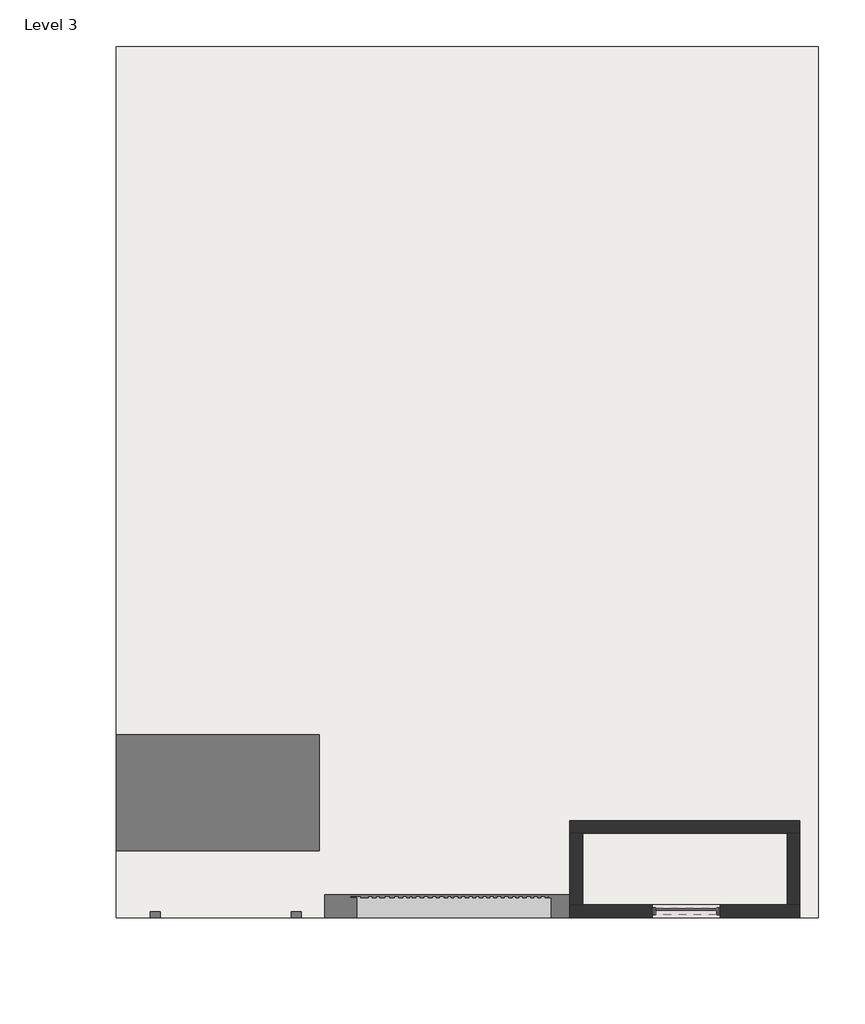
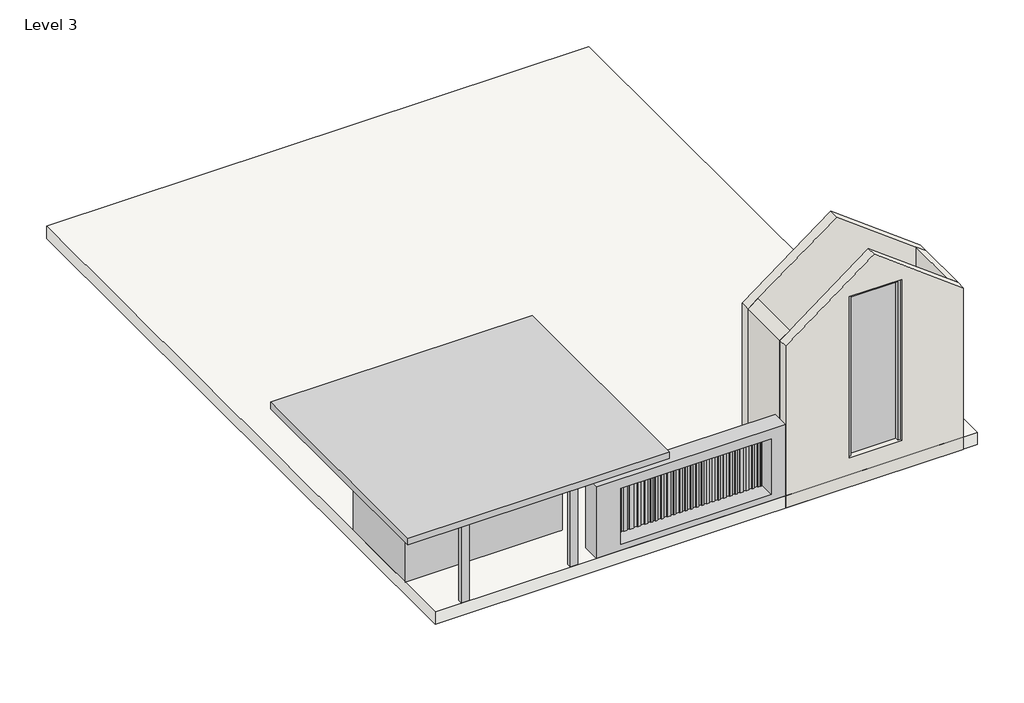
# One storey: 4 walls, 3 members, 1 plate, 1 proxy, 1 roof.
"""IFC4 building model written with IfcOpenShell, lengths in millimetres."""

from ifc_helpers import new_model, si_unit, frame, origin, place, context, project, spatial, polyline, outline, extrude, faceted_brep, transform, mapped, element, save
from components import generic_models_5_generic_models_5_ad9e1d00, member_97fca31a, member_273a15f2, system_panel_glazed_cfc6ab68

model = new_model("IFC4")

# Units and contexts
model_context = context("Model", 3, world=origin())
ifc_project = project(units=[si_unit("LENGTHUNIT", "METRE", prefix="MILLI")], contexts=[model_context])

# Site, building, storey
site = spatial("IfcSite", under=ifc_project)
building = spatial("IfcBuilding", under=site)
storey = spatial("IfcBuildingStorey", under=building, Name="Level 3", Elevation=6096.0)

# Proxy
placement = place(None, origin())
generic_models_5_generic_models_5_shape = generic_models_5_generic_models_5_ad9e1d00(model_context)
element("IfcBuildingElementProxy", 1, Name="Generic Models 5 : Generic Models 5", ObjectType="Generic Models 5 : Generic Models 5", at=placement, inside=storey, context=model_context, shape_type="MappedRepresentation", body=[
    mapped(generic_models_5_generic_models_5_shape, transform((0.0, 0.0, 0.0), x_axis=(1.0, 0.0, 0.0), y_axis=(0.0, 1.0, 0.0), z_axis=(0.0, 0.0, 1.0))),
])

# Members
member_shape = member_97fca31a(model_context)
element("IfcMember", 2, ObjectType="Rectangular Mullion : 2.5\" x 5\" rectangular", at=placement, inside=storey, context=model_context, shape_type="MappedRepresentation", body=[
    mapped(member_shape, transform((-12184.4451697, -14789.9171312, 10792.4603999), x_axis=(-1.0, 0.0, 0.0), y_axis=(0.0, -1.0, 0.0), z_axis=(0.0, 0.0, 1.0))),
])
member_2_shape = member_273a15f2(model_context)
element("IfcMember", 3, ObjectType="Rectangular Mullion : 2.5\" x 5\" rectangular", at=placement, inside=storey, context=model_context, shape_type="MappedRepresentation", body=[
    mapped(member_2_shape, transform((-11028.7451697, -14789.9171312, 10792.4603999), x_axis=(0.0, 0.0, 1.0), y_axis=(0.0, -1.0, 0.0), z_axis=(1.0, 0.0, 0.0))),
])
element("IfcMember", 4, ObjectType="Rectangular Mullion : 2.5\" x 5\" rectangular", at=placement, inside=storey, context=model_context, shape_type="MappedRepresentation", body=[
    mapped(member_shape, transform((-10965.2451697, -14789.9171312, 6813.0609972), x_axis=(1.0, 0.0, 0.0), y_axis=(0.0, -1.0, 0.0), z_axis=(0.0, 0.0, -1.0))),
])

# Plate
system_panel_glazed_shape = system_panel_glazed_cfc6ab68(model_context)
element("IfcPlate", 5, ObjectType="System Panel : Glazed", at=placement, inside=storey, context=model_context, shape_type="MappedRepresentation", body=[
    mapped(system_panel_glazed_shape, transform((-11574.8451697, -14789.9171312, 6813.0609972), x_axis=(1.0, 0.0, 0.0), y_axis=(0.0, 1.0, 0.0), z_axis=(0.0, 0.0, 1.0))),
])

# Roof
element("IfcRoof", 6, ObjectType="Generic - 12\"", at=placement, inside=storey, context=model_context, shape_type="SweptSolid", body=[
    extrude(outline(polyline([(-21845.6161422, 792.9828688), (-9196.4161422, 792.9828688), (-9196.4161422, -14904.2171312), (-21845.6161422, -14904.2171312), (-21845.6161422, 792.9828688)])), frame((0.0, 0.0, 6096.0), z_axis=(0.0, 0.0, 1.0), x_axis=(1.0, 0.0, 0.0)), (0.0, 0.0, 1.0), 304.8),
])

# Walls
element("IfcWall", 7, ObjectType="9\"", at=placement, inside=storey, context=model_context, shape_type="Brep", body=[
    faceted_brep([(-9528.1904814, -13160.519515, 6096.0), (-13670.3451697, -13160.519515, 6096.0), (-13670.3451697, -13160.519515, 10093.0339489), (-11606.7483033, -13160.519515, 11640.7315987), (-9528.1904814, -13160.519515, 10081.8132324), (-9528.1904814, -13389.119515, 6096.0), (-9528.1904814, -13389.119515, 10081.8132324), (-9756.7904814, -13389.119515, 10253.2632324), (-11606.7483033, -13389.119515, 11640.7315987), (-13441.7451697, -13389.119515, 10264.4839489), (-13670.3451697, -13389.119515, 10093.0339489), (-13670.3451697, -13389.119515, 6096.0), (-13441.7451697, -13389.119515, 6096.0), (-9756.7904814, -13389.119515, 6096.0)], [[[0, 1, 2, 3, 4]], [[5, 6, 7, 8, 9, 10, 11, 12, 13]], [[1, 0, 5, 13, 12, 11]], [[0, 4, 6, 5]], [[2, 1, 11, 10]], [[4, 3, 8, 7, 6]], [[3, 2, 10, 9, 8]]]),
])
element("IfcWall", 8, ObjectType="9\"", at=placement, inside=storey, context=model_context, shape_type="Brep", body=[
    faceted_brep([(-13670.3451697, -14904.2171312, 6096.0), (-9528.1904814, -14904.2171312, 6096.0), (-9528.1904814, -14904.2171312, 10081.8132324), (-11606.7483033, -14904.2171312, 11640.7315987), (-13670.3451697, -14904.2171312, 10093.0339489), (-12184.4451697, -14904.2171312, 6813.0609972), (-12184.4451697, -14904.2171312, 10792.4603999), (-10965.2451697, -14904.2171312, 10792.4603999), (-10965.2451697, -14904.2171312, 6813.0609972), (-9528.1904814, -14675.6171312, 6096.0), (-9756.7904814, -14675.6171312, 6096.0), (-13441.7451697, -14675.6171312, 6096.0), (-13670.3451697, -14675.6171312, 6096.0), (-13670.3451697, -14675.6171312, 10093.0339489), (-13441.7451697, -14675.6171312, 10264.4839489), (-11606.7483033, -14675.6171312, 11640.7315987), (-9756.7904814, -14675.6171312, 10253.2632324), (-9528.1904814, -14675.6171312, 10081.8132324), (-12184.4451697, -14675.6171312, 10792.4603999), (-12184.4451697, -14675.6171312, 6813.0609972), (-10965.2451697, -14675.6171312, 6813.0609972), (-10965.2451697, -14675.6171312, 10792.4603999)], [[[0, 1, 2, 3, 4], [5, 6, 7, 8]], [[9, 10, 11, 12, 13, 14, 15, 16, 17], [18, 19, 20, 21]], [[2, 1, 9, 17]], [[1, 0, 12, 11, 10, 9]], [[0, 4, 13, 12]], [[13, 4, 3, 15, 14]], [[2, 17, 16, 15, 3]], [[5, 19, 18, 6]], [[6, 18, 21, 7]], [[7, 21, 20, 8]], [[19, 5, 8, 20]]]),
])
element("IfcWall", 9, ObjectType="9\"", at=placement, inside=storey, context=model_context, shape_type="SweptSolid", body=[
    extrude(outline(polyline([(6096.0, -9528.1904814), (10081.8132324, -9528.1904814), (10253.2632324, -9756.7904814), (6096.0, -9756.7904814), (6096.0, -9528.1904814)])), frame((0.0, -14675.6171312, 0.0), z_axis=(0.0, 1.0, 0.0), x_axis=(0.0, 0.0, 1.0)), (0.0, 0.0, 1.0), 1286.4976162),
])
element("IfcWall", 10, ObjectType="9\"", at=placement, inside=storey, context=model_context, shape_type="SweptSolid", body=[
    extrude(outline(polyline([(6096.0, -13441.7451697), (10264.4839489, -13441.7451697), (10093.0339489, -13670.3451697), (6096.0, -13670.3451697), (6096.0, -13441.7451697)])), frame((0.0, -14675.6171312, 0.0), z_axis=(0.0, 1.0, 0.0), x_axis=(0.0, 0.0, 1.0)), (0.0, 0.0, 1.0), 1286.4976162),
])

save(model, "model.ifc")

# Revit data of these elements
# Type "Rectangular Mullion : 2.5\" x 5\" rectangular"
#   built-in parameter 1007304 = 0.416667 (stored number, unit not read)
#   built-in parameter 1007301 = 0.104167 (stored number, unit not read)
#   built-in parameter 1007300 = 0.104167 (stored number, unit not read)
# Type "System Panel : Glazed"
#   Construction Type Id = "GSP4R"
#   Analytic Construction = "1/8 in Pilkington single glazing"
#   Visual Light Transmittance = 0.9
#   Solar Heat Gain Coefficient = 0.86
#   Heat Transfer Coefficient (U) = 1.18115 BTU/(h·ft²·°F)
#   Define Thermal Properties by = 1
# Type "Generic - 12\""
#   Assembly Code = "B1020"
#   Layers, outside or top first: 1' - 0" no material (function 1)
# Type "9\""
#   Assembly Code = "B2010"
#   Layers, outside or top first: 0' - 9" no material (function 1)
# Element 1 (IfcBuildingElementProxy, "Generic Models 5 : Generic Models 5")
#   Phase Created = New Construction
# Elements 2, 3, 4 (IfcMember, "Rectangular Mullion : 2.5\" x 5\" rectangular")
#   Phase Created = New Construction
#   Materials on its faces: "Aluminum"
# Element 5 (IfcPlate, "System Panel : Glazed")
#   Phase Created = New Construction
#   Materials on its faces: "Glass"
# Element 6 (IfcRoof, "Generic - 12\"")
#   built-in parameter 1001705 = 21 (stored number, unit not read)
#   built-in parameter 1001710 = 33615
#   Phase Created = New Construction
#   Materials on its faces: "Default Roof"
# Elements 7, 8, 9, 10 (IfcWall, "9\"")
#   Top Offset = 0' - 0"
#   Base Offset = 0' - 0"
#   Unconnected Height = 10' - 0"
#   wall height = 10' - 0"
#   Phase Created = New Construction
#   Base Constraint = Level 3
#   Materials on its faces: "Default Wall"
# Materials
#   "Aluminum": class "Metal", colour RGB 247 247 247, transparency 0, Description = "Aluminum 6061", Cost = 0
#   "Glass": class "Glass", colour RGB 0 128 192, transparency 0.75, Description = "Soda Lime Glass", Cost = 0
#   "Default Roof": colour RGB 88 101 114, transparency 0, Cost = 0
#   "Default Wall": colour RGB 128 128 128, transparency 0, Cost = 0
